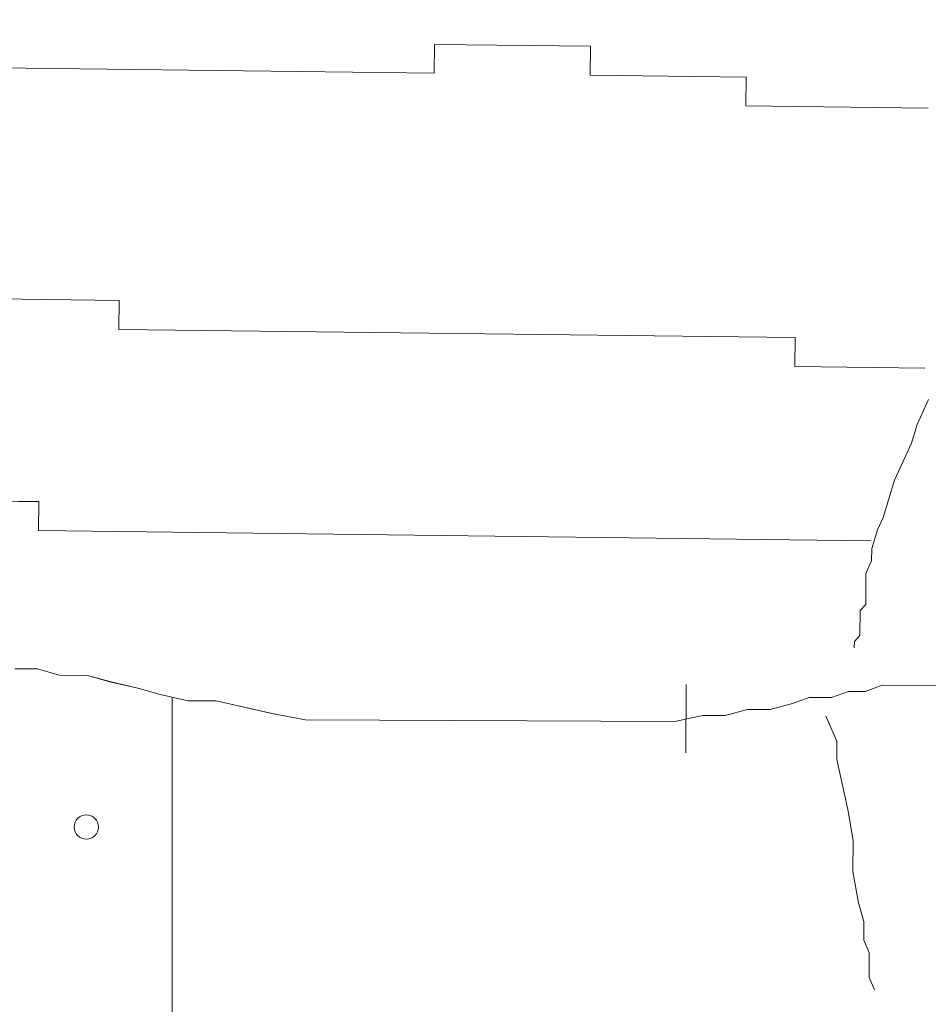
# Model space of a CAD drawing. Units: inches. Extents: x -466983 to 1020, y 324 to 318697.
# Tile 79 of 97: x 656.235 to 660.579, y 939.297 to 944.006. Entities that reach past the tile are written whole.
import ezdxf

# ---------------------------------------------------------------- set-up
doc = ezdxf.new("R2010")
doc.units = ezdxf.units.IN
doc.header["$MEASUREMENT"] = 0
doc.layers.add('A-FLOR-PATT', color=252, linetype='Continuous', lineweight=13)
doc.layers.add('A-FURN', color=8, linetype='Continuous', lineweight=18)

# ---------------------------------------------------------------- blocks, each defined once
blk = doc.blocks.new('L Shaped Sofa')
at = {"ltscale": 2}
for p, q in [((2394.7123, 747.2551), (2394.7123, 765.179)), ((2388.6357, 749.7), (2388.5876, 749.8086)), ((2388.6344, 749.4831), (2388.6357, 749.7)), ((2388.6826, 749.3745), (2388.6344, 749.4831)), ((2388.6816, 749.2118), (2388.6826, 749.3745)), ((2388.7294, 749.0489), (2388.6816, 749.2118)), ((2388.7765, 748.7776), (2388.7294, 749.0489)), ((2388.7748, 748.5065), (2388.7765, 748.7776)), ((2388.822, 748.2352), (2388.7748, 748.5065)), ((2388.9169, 747.801), (2388.822, 748.2352)), ((2388.9159, 747.6384), (2388.9169, 747.801)), ((2390.234, 747.7406), (2390.2304, 747.1443)), ((2389.0122, 747.4211), (2388.9159, 747.6384)), ((2390.0857, 747.416), (2390.33, 747.4691)), ((2390.33, 747.4691), (2393.5504, 747.454)), ((2393.5504, 747.454), (2393.8429, 747.3984)), ((2389.3043, 747.3113), (2389.4998, 747.3646)), ((2389.4998, 747.3646), (2389.695, 747.3637)), ((2389.695, 747.3637), (2389.8905, 747.417)), ((2389.8905, 747.417), (2390.0857, 747.416)), ((2393.8429, 747.3984), (2394.3302, 747.2877)), ((2389.1576, 747.2577), (2389.3043, 747.3113)), ((2394.3302, 747.2877), (2394.5741, 747.2865)), ((2394.5741, 747.2865), (2394.8178, 747.2312)), ((2388.5226, 747.1523), (2388.6693, 747.2058)), ((2388.6693, 747.2058), (2388.8157, 747.2051)), ((2388.8157, 747.2051), (2388.9624, 747.2587)), ((2388.9624, 747.2587), (2389.1576, 747.2577)), ((2394.8178, 747.2312), (2395.0126, 747.176)), ((2395.0126, 747.176), (2395.2563, 747.1207)), ((2387.3515, 747.1578), (2388.5226, 747.1523)), ((2395.2563, 747.1207), (2395.4511, 747.0656)), ((2395.4511, 747.0656), (2395.6951, 747.0644)), ((2395.6951, 747.0644), (2395.89, 747.0093)), ((2395.89, 747.0093), (2396.0851, 747.0084)), ((2388.7151, 746.7176), (2388.7642, 746.7716)), ((2388.7642, 746.7716), (2388.7645, 746.8258)), ((2388.7138, 746.5008), (2388.7151, 746.7176)), ((2388.6646, 746.4468), (2388.7138, 746.5008)), ((2388.663, 746.1757), (2388.6646, 746.4468)), ((2388.6135, 746.0675), (2388.663, 746.1757)), ((2388.6128, 745.9591), (2388.6135, 746.0675)), ((2388.5631, 745.7967), (2388.6128, 745.9591)), ((2388.6215, 745.891), (2395.8803, 745.8023)), ((2395.8803, 745.8023), (2395.8772, 745.5504)), ((2388.5136, 745.6885), (2388.5631, 745.7967)), ((2388.414, 745.3636), (2388.5136, 745.6885)), ((2395.8772, 745.5504), (2397.2382, 745.5337)), ((2388.2656, 745.039), (2388.414, 745.3636)), ((2388.2158, 744.8766), (2388.2656, 745.039)), ((2388.1169, 744.6602), (2388.2158, 744.8766)), ((2388.1494, 744.385), (2389.2836, 744.3712)), ((2389.2836, 744.3712), (2389.2805, 744.1193)), ((2389.2805, 744.1193), (2395.1782, 744.0472)), ((2395.1782, 744.0472), (2395.1752, 743.7953)), ((2395.1752, 743.7953), (2396.3094, 743.7814)), ((2388.1217, 742.1178), (2389.7096, 742.0984)), ((2389.7096, 742.0984), (2389.7065, 741.8465)), ((2389.7065, 741.8465), (2391.0675, 741.8299)), ((2391.0675, 741.8299), (2391.0644, 741.578)), ((2392.4254, 741.5613), (2392.4285, 741.8133)), ((2392.4285, 741.8133), (2397.6457, 741.7495)), ((2391.0644, 741.578), (2392.4254, 741.5613))]:
    blk.add_line(p, q, dxfattribs=at)
for start, end in [(90, 270), (270, 90)]:
    blk.add_arc((2395.4627, 748.3889), 0.1062, start, end, dxfattribs=at)

msp = doc.modelspace()

# ---------------------------------------------------------------- hatches: boundary and pattern name
at = {"layer": 'A-FLOR-PATT', "transparency": 33554572}
h = msp.add_hatch(dxfattribs=at)
h.set_pattern_fill('ANSI37', color=256, scale=30)
h.set_pattern_definition([(45, (-1212.4137, -290.035), (-2.6516504, 2.6516504), []), (135, (-1212.4137, -290.035), (-2.6516504, -2.6516504), [])])
h.paths.add_polyline_path([(901.8057, 1075.9377), (900.6144, 1075.9377), (900.6144, 1065.3856), (899.391, 1065.3856), (898.0911, 1065.3856), (892.8356, 1058.7098, -0.258377), (892.1875, 1058.3509), (879.9848, 1058.3509, -0.20177), (879.4382, 1058.5808), (874.0812, 1065.3856), (872.7813, 1065.3856), (871.5579, 1065.3856), (871.5579, 1075.9377), (813.8057, 1075.9377), (813.8057, 1044.7922), (832.3947, 1044.7922, -0.394795), (848.6602, 1028.5356), (848.6602, 1009.9377), (901.8057, 1009.9377), (901.8057, 1015.9377), (901.3057, 1015.9377), (871.3057, 1015.9377), (871.3057, 1017.2502), (871.3344, 1017.2502, -0.401453), (901.3057, 1045.9377), (901.8057, 1045.9377)])
edge = h.paths.add_edge_path(flags=16)
edge.add_line((847.7731, 1068.9486), (847.7731, 1073.7088))
edge.add_arc((849.2269, 1073.7088), 1.4538, 90, 180, ccw=False)
edge.add_line((849.2269, 1075.1627), (864.4921, 1075.1627))
edge.add_arc((864.4921, 1073.7088), 1.4538, 0, 90, ccw=False)
edge.add_line((865.9459, 1073.7088), (865.9459, 1069.0035))
edge.add_arc((832.6447, 1068.9761), 33.3012, -20.61234, 0.04725, ccw=False)
edge.add_ellipse((856.8595, 1058.48), major_axis=(0, 10.2131), ratio=0.6859192, start_angle=100.00884, end_angle=259.99116, ccw=False)
edge.add_arc((881.0742, 1068.9761), 33.3012, 180.04725, 200.61234, ccw=False)
h.paths.add_polyline_path([(853.1456, 1066.4815), (853.1456, 1066.4534), (853.1463, 1066.4534, 0.433107), (852.9166, 1066.6849), (852.9166, 1066.4534), (853.1456, 1066.4534), (853.1456, 1066.4815), (853.088, 1066.6122, 0.697939), (852.6995, 1066.4534), (852.7003, 1066.4534), (852.7003, 1066.4815), (852.9166, 1067.0012), (852.9166, 1066.6849, -0.396254)], flags=0)
h.paths.add_polyline_path([(861.0187, 1066.4815), (861.0187, 1066.4534), (861.0194, 1066.4534, 0.416404), (860.8024, 1066.6849), (860.8024, 1066.4534), (861.0187, 1066.4534), (861.0187, 1066.4815), (860.9672, 1066.6053, 0.713344), (860.5726, 1066.4534), (860.5734, 1066.4534), (860.5734, 1066.4815), (860.8024, 1067.0012), (860.8024, 1066.6849, -0.379973)], flags=0)
edge = h.paths.add_edge_path(flags=0)
edge.add_spline(control_points=[(861.1298, 1065.7855), (861.4661, 1065.2478), (861.6134, 1065.0161), (861.9833, 1064.3736), (862.1924, 1063.9443), (862.5614, 1063.0391), (862.7212, 1062.5633), (862.9865, 1061.5781), (863.092, 1061.0689), (863.2452, 1060.031), (863.293, 1059.5025), (863.3295, 1058.4409), (863.3181, 1057.9078), (863.2366, 1056.8518), (863.1664, 1056.3289), (862.9695, 1055.308), (862.8427, 1054.8099), (862.5365, 1053.8522), (862.3571, 1053.3927), (861.9514, 1052.5249), (861.7251, 1052.1166), (861.233, 1051.3622), (860.9672, 1051.0162), (860.4048, 1050.3949), (860.1082, 1050.1197), (859.4937, 1049.6461), (859.1758, 1049.4476), (858.5276, 1049.1299), (858.1973, 1049.0107), (857.5315, 1048.8518), (857.1959, 1048.8121), (856.5249, 1048.812), (856.1894, 1048.8515), (855.5236, 1049.0101), (855.1933, 1049.1291), (854.545, 1049.4465), (854.2271, 1049.6449), (853.6124, 1050.1183), (853.3158, 1050.3933), (852.7533, 1051.0143), (852.4874, 1051.3602), (851.9952, 1052.1144), (851.7688, 1052.5225), (851.3629, 1053.3902), (851.1834, 1053.8496), (850.877, 1054.8071), (850.7501, 1055.3051), (850.553, 1056.326), (850.4827, 1056.8488), (850.401, 1057.9048), (850.3895, 1058.4379), (850.4257, 1059.4995), (850.4734, 1060.0281), (850.6265, 1061.066), (850.7318, 1061.5753), (850.9969, 1062.5605), (851.1567, 1063.0365), (851.5254, 1063.9418), (851.7345, 1064.3712), (852.1056, 1065.0164), (852.2544, 1065.2503), (852.6082, 1065.7335)], knot_values=[3.915332, 3.915332, 3.915332, 3.915332, 4.013468, 4.013468, 4.175532, 4.175532, 4.337596, 4.337596, 4.49966, 4.49966, 4.661724, 4.661724, 4.823788, 4.823788, 4.985852, 4.985852, 5.147916, 5.147916, 5.30998, 5.30998, 5.472044, 5.472044, 5.634109, 5.634109, 5.796173, 5.796173, 5.958237, 5.958237, 6.120301, 6.120301, 6.282365, 6.282365, 6.444429, 6.444429, 6.606493, 6.606493, 6.768557, 6.768557, 6.930621, 6.930621, 7.092685, 7.092685, 7.254749, 7.254749, 7.416813, 7.416813, 7.578878, 7.578878, 7.740942, 7.740942, 7.903006, 7.903006, 8.06507, 8.06507, 8.227134, 8.227134, 8.389198, 8.389198, 8.551262, 8.551262, 8.65037, 8.65037, 8.65037, 8.65037], degree=3, periodic=0)
edge.add_line((852.6421, 1065.7855), (861.1298, 1065.7855))
edge = h.paths.add_edge_path(flags=0)
edge.add_ellipse((856.8496, 1057.7432), major_axis=(0, 7.7921), ratio=0.687861, start_angle=0, end_angle=360)
h.paths.add_polyline_path([(848.8634, 1069.3891), (848.8634, 1073.9605, -0.414214), (849.9538, 1075.0508), (863.7652, 1075.0508, -0.414214), (864.8555, 1073.9605), (864.8555, 1069.3891, -0.388936), (864.5237, 1069.027, -0.043561), (849.1953, 1069.027, -0.388936)], flags=0)
h.paths.add_polyline_path([(853.1006, 1068.1122, -1), (852.6775, 1068.1122, -1)], flags=0)
edge = h.paths.add_edge_path(flags=0)
edge.add_ellipse((856.8595, 1057.3378), major_axis=(0, 2.207), ratio=0.657164, start_angle=0, end_angle=360)
h.paths.add_polyline_path([(861.0415, 1068.1122, -1), (860.6184, 1068.1122, -1)], flags=0)
edge = h.paths.add_edge_path()
edge.add_line((573.9537, 1057.3412), (573.9537, 1075.9377))
edge.add_line((573.9537, 1075.9377), (558.7308, 1075.9377))
edge.add_line((558.7308, 1075.9377), (558.7308, 1065.3856))
edge.add_line((558.7308, 1065.3856), (557.5074, 1065.3856))
edge.add_line((557.5074, 1065.3856), (556.2075, 1065.3856))
edge.add_line((556.2075, 1065.3856), (550.952, 1058.7098))
edge.add_arc((550.3039, 1059.1155), 0.7646, 270, 327.9483, ccw=False)
edge.add_line((550.3039, 1058.3509), (538.1012, 1058.3509))
edge.add_arc((538.1012, 1059.1155), 0.7646, 224.3704, 270, ccw=False)
edge.add_line((537.5546, 1058.5808), (532.1976, 1065.3856))
edge.add_line((532.1976, 1065.3856), (530.8977, 1065.3856))
edge.add_line((530.8977, 1065.3856), (529.6743, 1065.3856))
edge.add_line((529.6743, 1065.3856), (529.6743, 1075.9377))
edge.add_line((529.6743, 1075.9377), (520.8057, 1075.9377))
edge.add_line((520.8057, 1075.9377), (520.8057, 1045.9377))
edge.add_line((520.8057, 1045.9377), (521.3057, 1045.9377))
edge.add_arc((521.3057, 1015.9377), 30, 2.50749, 90, ccw=False)
edge.add_line((551.277, 1017.2502), (551.3057, 1017.2502))
edge.add_line((551.3057, 1017.2502), (551.3057, 1015.9377))
edge.add_line((551.3057, 1015.9377), (520.8057, 1015.9377))
edge.add_line((520.8057, 1015.9377), (520.8057, 1009.9377))
edge.add_line((520.8057, 1009.9377), (559.1913, 1010.4022))
edge.add_arc((559.1913, 1011.856), 1.4538, 180, 270, ccw=False)
edge.add_line((557.7375, 1011.856), (557.7375, 1016.5613))
edge.add_arc((591.0386, 1016.5888), 33.3012, 159.38766, 180.04725, ccw=False)
edge.add_ellipse((566.8239, 1027.0848), major_axis=(0, 10.2131), ratio=0.6859192, start_angle=280.00884, end_angle=439.99116, ccw=False)
edge.add_arc((542.6091, 1016.5888), 33.3012, 0.04725, 20.61234, ccw=False)
edge.add_line((575.9103, 1016.6162), (575.9103, 1011.856))
edge.add_arc((574.4565, 1011.856), 1.4538, -90, 0, ccw=False)
edge.add_line((574.4565, 1010.4022), (608.8057, 1009.9377))
edge.add_line((608.8057, 1009.9377), (608.8057, 1041.0857))
edge.add_line((608.8057, 1041.0857), (590.2179, 1041.0857))
edge.add_arc((590.775, 1057.9074), 16.8309, 181.92775, 268.10321, ccw=False)
edge = h.paths.add_edge_path()
edge.add_ellipse((494.2443, 583.6204), major_axis=(0, 10.2131), ratio=0.6859192, start_angle=280.00884, end_angle=439.99116, ccw=False)
edge.add_arc((470.0296, 573.1243), 33.3012, 0.04725, 20.61234, ccw=False)
edge.add_line((503.3307, 573.1518), (503.3307, 568.3916))
edge.add_arc((501.8769, 568.3916), 1.4538, -90, 0, ccw=False)
edge.add_line((501.8769, 566.9377), (539.8057, 566.9377))
edge.add_line((539.8057, 566.9377), (539.8057, 572.9377))
edge.add_line((539.8057, 572.9377), (539.3057, 572.9377))
edge.add_line((539.3057, 572.9377), (509.3057, 572.9377))
edge.add_line((509.3057, 572.9377), (509.3057, 574.2502))
edge.add_line((509.3057, 574.2502), (509.3344, 574.2502))
edge.add_arc((539.3057, 572.9377), 30, 90, 177.49251, ccw=False)
edge.add_line((539.3057, 602.9377), (539.8057, 602.9377))
edge.add_line((539.8057, 602.9377), (539.8057, 626.9377))
edge.add_line((539.8057, 626.9377), (531.7718, 626.9377))
edge.add_line((531.7718, 626.9377), (531.7718, 616.3856))
edge.add_line((531.7718, 616.3856), (530.5484, 616.3856))
edge.add_line((530.5484, 616.3856), (529.2485, 616.3856))
edge.add_line((529.2485, 616.3856), (523.7105, 609.3509))
edge.add_line((523.7105, 609.3509), (510.7766, 609.3509))
edge.add_line((510.7766, 609.3509), (505.2386, 616.3856))
edge.add_line((505.2386, 616.3856), (503.9387, 616.3856))
edge.add_line((503.9387, 616.3856), (502.7153, 616.3856))
edge.add_line((502.7153, 616.3856), (502.7153, 626.9377))
edge.add_line((502.7153, 626.9377), (481.6983, 626.9377))
edge.add_line((481.6983, 626.9377), (481.6983, 610.995))
edge.add_arc((467.2703, 611.4728), 14.4359, 271.92775, 358.10321, ccw=False)
edge.add_line((467.7559, 597.0451), (451.8057, 597.0451))
edge.add_line((451.8057, 597.0451), (451.8057, 584.4035))
edge.add_line((451.8057, 584.4035), (451.8057, 566.9377))
edge.add_line((451.8057, 566.9377), (486.6117, 566.9377))
edge.add_arc((486.6117, 568.3916), 1.4538, 180, 270, ccw=False)
edge.add_line((485.1579, 568.3916), (485.1579, 573.0969))
edge.add_arc((518.4591, 573.1243), 33.3012, 159.38766, 180.04725, ccw=False)
h.paths.add_polyline_path([(836.2609, 1020.7328), (879.8898, 1020.7328), (879.8898, 1039.3902), (836.2609, 1039.3902)], flags=25)
h.paths.add_polyline_path([(549.9851, 1036.7492), (593.614, 1036.7492), (593.614, 1055.4065), (549.9851, 1055.4065)], flags=24)
h.paths.add_polyline_path([(475.123, 595.5959), (518.752, 595.5959), (518.752, 614.2532), (475.123, 614.2532)], flags=24)
h = msp.add_hatch(dxfattribs=at)
h.set_pattern_fill('ANSI37', color=256, scale=20)
h.set_pattern_definition([(45, (-1212.4137, -290.035), (-1.767767, 1.767767), []), (135, (-1212.4137, -290.035), (-1.767767, -1.767767), [])])
h.paths.add_polyline_path([(809.8057, 870.9377), (809.8057, 888.1519), (806.9985, 888.1519), (802.6624, 888.1519), (789.3832, 888.1519), (786.2846, 888.1519, -0.414214), (785.4991, 888.9374), (785.4991, 900.1959), (785.4991, 908.4696, -0.414214), (786.8082, 909.7787, -0.414214), (785.4991, 911.0878), (785.4991, 929.1015, -0.414214), (786.8082, 930.4106, -0.414214), (785.4991, 931.7197), (785.4991, 931.9039, -0.414214), (784.19, 930.5948), (766.7223, 930.5948, -0.412359), (765.4132, 931.8956, -0.413741), (764.1145, 930.5782), (744.5781, 930.422, -0.416556), (743.7864, 931.2075), (743.7864, 933.5153), (742.2154, 933.5153), (742.2154, 952.024, -0.001344), (743.7864, 952.1998), (743.7864, 953.9377), (678.5915, 953.9377), (678.5915, 951.1305), (678.5915, 946.7945), (678.5915, 933.5153), (678.5915, 930.4166, -0.414214), (677.806, 929.6312), (666.5475, 929.6312), (658.2738, 929.6312, -0.414214), (656.9647, 930.9403, -0.414214), (655.6556, 929.6312), (637.6419, 929.6312, -0.414214), (636.3328, 930.9403, -0.414214), (635.0237, 929.6312), (634.8395, 929.6312, -0.414214), (636.1486, 928.322), (636.1486, 910.8544, -0.412359), (634.8478, 909.5452, -0.413741), (636.1653, 908.2466), (636.3214, 888.7102, -0.416556), (635.5359, 887.9184), (633.2281, 887.9184), (633.2281, 886.3475), (614.7194, 886.3475, -0.001344), (614.5436, 887.9184), (612.8057, 887.9184), (612.8057, 834.9377), (612.8057, 752.9377), (612.8057, 748.9377), (612.8057, 697.9377), (654.8057, 697.9377), (654.8057, 701.9377), (715.8057, 701.9377), (715.8057, 737.4353), (774.2918, 737.4353), (774.2918, 795.9377), (809.8057, 795.9377)])
h.paths.add_polyline_path([(679.2761, 849.5757, 0.102523), (682.1475, 849.2608, -0.080461), (694.5428, 849.7725, -0.283899), (694.4822, 849.0082, 0.136605), (694.4068, 848.8103, -0.030441), (694.5428, 846.8929), (694.5428, 842.6198), (694.5428, 838.3466, -0.028219), (694.4246, 836.5684), (694.425, 836.5684, 0.196187), (694.4456, 836.2708, -0.302897), (694.5428, 835.467, -0.080461), (682.1475, 835.9787, 0.102523), (679.2761, 835.6638, -0.58611), (678.6457, 836.0169), (678.6457, 849.2227, -0.58611)], flags=16)
h.paths.add_polyline_path([(679.5173, 848.6515, 0.699597), (679.476, 848.6342, 1.20716), (679.1935, 848.7422, 0.010621)], flags=0)
h.paths.add_polyline_path([(679.4923, 836.5608, -0.013798), (679.9178, 836.6594, -0.071703), (682.8533, 837.1434, -0.165743), (682.1665, 839.1006), (682.1665, 842.6094), (682.1665, 846.0603, -0.240616), (683.4733, 848.6767, -0.068263), (693.9295, 849.0082), (693.7875, 848.7083), (693.7875, 849.0228, 0.067332), (683.4733, 848.6767, 0.240616), (682.1665, 846.0603), (682.1665, 842.6094), (682.1665, 839.1006, 0.23459), (683.461, 836.5513, 0.068093), (693.7875, 836.1955), (693.7875, 836.5104), (693.9296, 836.2102, -0.077215), (682.2421, 836.7815, 0.086627), (679.5283, 836.5701, -0.628402), (679.5029, 836.5735), (679.5029, 836.6071, 0.910458)], flags=0)
h.paths.add_polyline_path([(679.476, 848.6364), (679.2069, 848.647), (679.2069, 836.5718, 0.913566), (679.3645, 836.5861), (679.476, 836.5824)], flags=0)
h.paths.add_polyline_path([(679.2761, 829.8604, 0.102523), (682.1475, 829.5455, -0.080461), (694.5428, 830.0572, -0.283899), (694.4822, 829.2929, 0.136605), (694.4068, 829.095, -0.030441), (694.5428, 827.1776), (694.5428, 822.9045), (694.5428, 818.6314, -0.028219), (694.4246, 816.8531), (694.425, 816.8532, 0.196187), (694.4456, 816.5555, -0.302897), (694.5428, 815.7517, -0.080461), (682.1475, 816.2635, 0.102523), (679.2761, 815.9485, -0.58611), (678.6457, 816.3016), (678.6457, 829.5074, -0.58611)], flags=16)
h.paths.add_polyline_path([(679.5173, 828.9362, 0.699597), (679.476, 828.9189, 1.20716), (679.1935, 829.0269, 0.010621)], flags=0)
h.paths.add_polyline_path([(679.4923, 816.8456, -0.013798), (679.9178, 816.9441, -0.071703), (682.8533, 817.4281, -0.165743), (682.1665, 819.3853), (682.1665, 822.8941), (682.1665, 826.345, -0.240616), (683.4733, 828.9614, -0.068263), (693.9295, 829.2929), (693.7875, 828.9931), (693.7875, 829.3076, 0.067332), (683.4733, 828.9614, 0.240616), (682.1665, 826.345), (682.1665, 822.8941), (682.1665, 819.3853, 0.23459), (683.461, 816.836, 0.068093), (693.7875, 816.4802), (693.7875, 816.7952), (693.9296, 816.4949, -0.077215), (682.2421, 817.0662, 0.086627), (679.5283, 816.8549, -0.628402), (679.5029, 816.8582), (679.5029, 816.8918, 0.910458)], flags=0)
h.paths.add_polyline_path([(679.476, 828.9211), (679.2069, 828.9317), (679.2069, 816.8565, 0.913566), (679.3645, 816.8708), (679.476, 816.8671)], flags=0)
h.paths.add_polyline_path([(679.2761, 810.1451, 0.102523), (682.1475, 809.8302, -0.080461), (694.5428, 810.342, -0.3023), (694.4466, 809.5394, 0.10023), (694.4058, 809.3878, -0.03057), (694.5428, 807.4623), (694.5428, 803.1892), (694.5428, 798.9161, -0.03057), (694.4058, 796.9906, 0.10023), (694.4466, 796.839, -0.3023), (694.5428, 796.0365, -0.080461), (682.1475, 796.5482, 0.102523), (679.2761, 796.2333, -0.58611), (678.6457, 796.5863), (678.6457, 809.7921, -0.58611)], flags=16)
h.paths.add_polyline_path([(679.5173, 809.2417, 0.699597), (679.476, 809.2244, 1.20716), (679.1935, 809.3324, 0.010621)], flags=0)
h.paths.add_polyline_path([(679.4923, 797.151, -0.013798), (679.9178, 797.2496, -0.071703), (682.8533, 797.7336, -0.165743), (682.1665, 799.6908), (682.1665, 803.1996), (682.1665, 806.6505, -0.239349), (683.461, 809.2577, -0.072465), (694.4468, 809.5405, 0.197932), (694.425, 809.2405), (693.7875, 809.2985), (693.7875, 809.6135, 0.068093), (683.461, 809.2577, 0.239349), (682.1665, 806.6505), (682.1665, 803.1996), (682.1665, 799.6908, 0.235854), (683.4733, 797.1323, 0.067332), (693.7875, 796.7861), (693.7875, 797.1006), (694.425, 797.1586, 0.197932), (694.4468, 796.8586, -0.080419), (682.1557, 797.3795, 0.083867), (679.5283, 797.1603, -0.628402), (679.5029, 797.1637), (679.5029, 797.1973, 0.910458)], flags=0)
h.paths.add_polyline_path([(679.2069, 809.2372), (679.2069, 797.162, 0.913566), (679.3645, 797.1763), (679.476, 797.1726), (679.476, 809.2266)], flags=0)
h.paths.add_polyline_path([(695.3643, 853.2989), (728.2231, 853.2989), (728.2231, 771.1519), (695.3643, 771.1519)], flags=16)
h.paths.add_polyline_path([(696.0215, 852.6417), (727.5659, 852.6417), (727.5659, 771.809), (696.0215, 771.809)], flags=0)
h.paths.add_polyline_path([(679.2761, 788.7869, 0.102523), (682.1475, 788.472, -0.080461), (694.5428, 788.9837, -0.3023), (694.4466, 788.1812, 0.10023), (694.4058, 788.0296, -0.03057), (694.5428, 786.1041), (694.5428, 781.831), (694.5428, 777.5578, -0.03057), (694.4058, 775.6323, 0.10023), (694.4466, 775.4808, -0.3023), (694.5428, 774.6782, -0.080461), (682.1475, 775.19, 0.102523), (679.2761, 774.875, -0.58611), (678.6457, 775.2281), (678.6457, 788.4339, -0.58611)], flags=16)
h.paths.add_polyline_path([(679.5173, 787.8834, 0.699597), (679.476, 787.8662, 1.20716), (679.1935, 787.9742, 0.010621)], flags=0)
h.paths.add_polyline_path([(679.4923, 775.7928, -0.013798), (679.9178, 775.8914, -0.071703), (682.8533, 776.3753, -0.165743), (682.1665, 778.3325), (682.1665, 781.8414), (682.1665, 785.2922, -0.239349), (683.461, 787.8995, -0.072465), (694.4468, 788.1823, 0.197932), (694.425, 787.8823), (693.7875, 787.9403), (693.7875, 788.2553, 0.068093), (683.461, 787.8995, 0.239349), (682.1665, 785.2922), (682.1665, 781.8414), (682.1665, 778.3325, 0.235854), (683.4733, 775.7741, 0.067332), (693.7875, 775.4279), (693.7875, 775.7424), (694.425, 775.8004, 0.197932), (694.4468, 775.5004, -0.080419), (682.1557, 776.0212, 0.083867), (679.5283, 775.8021, -0.628402), (679.5029, 775.8054), (679.5029, 775.8391, 0.910458)], flags=0)
h.paths.add_polyline_path([(679.2069, 787.8789), (679.2069, 775.8038, 0.913566), (679.3645, 775.818), (679.476, 775.8144), (679.476, 787.8684)], flags=0)
h.paths.add_polyline_path([(704.641, 854.1204, -0.080461), (705.1527, 866.5157, 0.102523), (704.8378, 869.3871, -0.58611), (705.1908, 870.0174), (718.3966, 870.0174, -0.58611), (718.7496, 869.3871, 0.102523), (718.4347, 866.5157, -0.080461), (718.9465, 854.1204, -0.3023), (718.1439, 854.2166, 0.10023), (717.9924, 854.2574, -0.03057), (716.0668, 854.1204), (711.7937, 854.1204), (707.5206, 854.1204, -0.03057), (705.5951, 854.2574, 0.10023), (705.4435, 854.2166, -0.3023)], flags=16)
h.paths.add_polyline_path([(717.8462, 869.1459, 0.699597), (717.8289, 869.1872, 1.20716), (717.9369, 869.4697, 0.010621)], flags=0)
h.paths.add_polyline_path([(705.4631, 854.2164, -0.080419), (705.984, 866.5074, 0.083867), (705.7648, 869.1349, -0.628402), (705.7682, 869.1603), (705.8018, 869.1603, 0.910458), (705.7555, 869.1709, -0.013798), (705.8541, 868.7454, -0.071703), (706.3381, 865.8099, -0.165743), (708.2953, 866.4967), (711.8041, 866.4967), (715.255, 866.4967, -0.239349), (717.8622, 865.2022, -0.072465), (718.145, 854.2164, 0.197932), (717.845, 854.2382), (717.903, 854.8757), (718.218, 854.8757, 0.068093), (717.8622, 865.2022, 0.239349), (715.255, 866.4967), (711.8041, 866.4967), (708.2953, 866.4967, 0.235854), (705.7368, 865.1898, 0.067332), (705.3906, 854.8757), (705.7051, 854.8757), (705.7631, 854.2382, 0.197932)], flags=16)
h.paths.add_polyline_path([(705.7665, 869.4563, 0.913566), (705.7808, 869.2987), (705.7771, 869.1872), (717.8311, 869.1872), (717.8417, 869.4563)], flags=0)
h.paths.add_polyline_path([(729.0446, 842.6198), (729.0446, 846.8929, -0.03057), (729.1817, 848.8184, 0.10023), (729.1408, 848.9699, -0.3023), (729.0446, 849.7725, -0.080461), (741.4399, 849.2608, 0.102523), (744.3113, 849.5757, -0.58611), (744.9417, 849.2227), (744.9417, 836.0169, -0.58611), (744.3113, 835.6638, 0.102523), (741.4399, 835.9787, -0.080461), (729.0446, 835.467, -0.3023), (729.1408, 836.2696, 0.10023), (729.1817, 836.4211, -0.03057), (729.0446, 838.3466)], flags=16)
h.paths.add_polyline_path([(744.1115, 836.5846, 1.20716), (744.3939, 836.4766, 0.010621), (744.0701, 836.5673, 0.699597)], flags=0)
h.paths.add_polyline_path([(729.1407, 836.2684, 0.197932), (729.1624, 836.5684), (729.7999, 836.5104), (729.7999, 836.1955, 0.068093), (740.1264, 836.5513, 0.239349), (741.4209, 839.1585), (741.4209, 842.6094), (741.4209, 846.1182, 0.235854), (740.1141, 848.6767, 0.067332), (729.7999, 849.0228), (729.7999, 848.7083), (729.1624, 848.6503, 0.197932), (729.1407, 848.9504, -0.080419), (741.4317, 848.4295, 0.083867), (744.0591, 848.6486, -0.628402), (744.0845, 848.6453), (744.0845, 848.6117, 0.910458), (744.0951, 848.6579, -0.013798), (743.6696, 848.5594, -0.071703), (740.7341, 848.0754, -0.165743), (741.4209, 846.1182), (741.4209, 842.6094), (741.4209, 839.1585, -0.239349), (740.1264, 836.5513, -0.072465)], flags=0)
h.paths.add_polyline_path([(729.0446, 830.0572, -0.080461), (741.4399, 829.5455, 0.102523), (744.3113, 829.8604, -0.58611), (744.9417, 829.5074), (744.9417, 816.3016, -0.58611), (744.3113, 815.9485, 0.102523), (741.4399, 816.2635, -0.080461), (729.0446, 815.7517, -0.3023), (729.1408, 816.5543, 0.10023), (729.1817, 816.7058, -0.03057), (729.0446, 818.6314), (729.0446, 822.9045), (729.0446, 827.1776, -0.03057), (729.1817, 829.1031, 0.10023), (729.1408, 829.2547, -0.3023)], flags=16)
h.paths.add_polyline_path([(744.1115, 816.8693, 1.20716), (744.3939, 816.7613, 0.010621), (744.0701, 816.852, 0.699597)], flags=0)
h.paths.add_polyline_path([(729.1407, 829.2351, -0.080419), (741.4317, 828.7142, 0.083867), (744.0591, 828.9334, -0.628402), (744.0845, 828.93), (744.0845, 828.8964, 0.910458), (744.0951, 828.9427, -0.013798), (743.6696, 828.8441, -0.071703), (740.7341, 828.3601, -0.165743), (741.4209, 826.4029), (741.4209, 822.8941), (741.4209, 819.4432, -0.239349), (740.1264, 816.836, -0.072465), (729.1407, 816.5531, 0.197932), (729.1624, 816.8532), (729.7999, 816.7952), (729.7999, 816.4802, 0.068093), (740.1264, 816.836, 0.239349), (741.4209, 819.4432), (741.4209, 822.8941), (741.4209, 826.4029, 0.235854), (740.1141, 828.9614, 0.067332), (729.7999, 829.3076), (729.7999, 828.9931), (729.1624, 828.9351, 0.197932)], flags=16)
h.paths.add_polyline_path([(729.0446, 810.342, -0.080461), (741.4399, 809.8302, 0.102523), (744.3113, 810.1451, -0.58611), (744.9417, 809.7921), (744.9417, 796.5863, -0.58611), (744.3113, 796.2333, 0.102523), (741.4399, 796.5482, -0.080461), (729.0446, 796.0365, -0.283899), (729.1052, 796.8007, 0.136605), (729.1806, 796.9987, -0.030441), (729.0446, 798.9161), (729.0446, 803.1892), (729.0446, 807.4623, -0.028219), (729.1628, 809.2406), (729.1624, 809.2405, 0.196187), (729.1418, 809.5382, -0.302897)], flags=16)
h.paths.add_polyline_path([(744.1115, 797.1748, 1.20716), (744.3939, 797.0668, 0.010621), (744.0701, 797.1575, 0.699597)], flags=0)
h.paths.add_polyline_path([(741.3453, 809.0275, 0.086627), (744.0591, 809.2388, -0.628402), (744.0845, 809.2355), (744.0845, 809.2019, 0.910458), (744.0951, 809.2481, -0.013798), (743.6696, 809.1496, -0.071703), (740.7341, 808.6656, -0.165743), (741.4209, 806.7084), (741.4209, 803.1996), (741.4209, 799.7487, -0.240616), (740.1141, 797.1323, -0.068263), (729.658, 796.8008), (729.7999, 797.1006), (729.7999, 796.7861, 0.067332), (740.1141, 797.1323, 0.240616), (741.4209, 799.7487), (741.4209, 803.1996), (741.4209, 806.7084, 0.23459), (740.1264, 809.2577, 0.068093), (729.7999, 809.6135), (729.7999, 809.2985), (729.6578, 809.5988, -0.077215)], flags=0)
h.paths.add_polyline_path([(704.641, 770.3304, -0.283899), (705.4053, 770.2697, 0.136605), (705.6032, 770.1944, -0.030441), (707.5206, 770.3304), (711.7937, 770.3304), (716.0668, 770.3304, -0.028219), (717.8451, 770.2122), (717.845, 770.2126, 0.196187), (718.1427, 770.2331, -0.302897), (718.9465, 770.3304, -0.080461), (718.4347, 757.9351, 0.102523), (718.7496, 755.0637, -0.58611), (718.3966, 754.4333), (705.1908, 754.4333, -0.58611), (704.8378, 755.0637, 0.102523), (705.1527, 757.9351, -0.080461)], flags=16)
h.paths.add_polyline_path([(705.762, 755.3048, 0.699597), (705.7793, 755.2635, 1.20716), (705.6713, 754.9811, 0.010621)], flags=0)
h.paths.add_polyline_path([(705.4053, 769.717), (705.7051, 769.5751), (705.3906, 769.5751, 0.067332), (705.7368, 759.2609, 0.240616), (708.3532, 757.954), (711.8041, 757.954), (715.3129, 757.954, 0.23459), (717.8622, 759.2485, 0.068093), (718.218, 769.5751), (717.903, 769.5751), (718.2033, 769.7172, -0.077215), (717.632, 758.0297, 0.086627), (717.8433, 755.3159, -0.628402), (717.84, 755.2904), (717.8064, 755.2904, 0.910458), (717.8526, 755.2799, -0.013798), (717.7541, 755.7053, -0.071703), (717.2701, 758.6409, -0.165743), (715.3129, 757.954), (711.8041, 757.954), (708.3532, 757.954, -0.240616), (705.7368, 759.2609, -0.068263)], flags=0)
h.paths.add_polyline_path([(729.0446, 788.9837, -0.080461), (741.4399, 788.472, 0.102523), (744.3113, 788.7869, -0.58611), (744.9417, 788.4339), (744.9417, 775.2281, -0.58611), (744.3113, 774.875, 0.102523), (741.4399, 775.19, -0.080461), (729.0446, 774.6782, -0.283899), (729.1052, 775.4425, 0.136605), (729.1806, 775.6405, -0.030441), (729.0446, 777.5578), (729.0446, 781.831), (729.0446, 786.1041, -0.028219), (729.1628, 787.8823), (729.1624, 787.8823, 0.196187), (729.1418, 788.1799, -0.302897)], flags=16)
h.paths.add_polyline_path([(744.1115, 775.8165, 1.20716), (744.3939, 775.7086, 0.010621), (744.0701, 775.7993, 0.699597)], flags=0)
h.paths.add_polyline_path([(741.3453, 787.6692, 0.086627), (744.0591, 787.8806, -0.628402), (744.0845, 787.8773), (744.0845, 787.8437, 0.910458), (744.0951, 787.8899, -0.013798), (743.6696, 787.7913, -0.071703), (740.7341, 787.3074, -0.165743), (741.4209, 785.3502), (741.4209, 781.8414), (741.4209, 778.3905, -0.240616), (740.1141, 775.7741, -0.068263), (729.658, 775.4425), (729.7999, 775.7424), (729.7999, 775.4279, 0.067332), (740.1141, 775.7741, 0.240616), (741.4209, 778.3905), (741.4209, 781.8414), (741.4209, 785.3502, 0.23459), (740.1264, 787.8995, 0.068093), (729.7999, 788.2553), (729.7999, 787.9403), (729.6578, 788.2405, -0.077215)], flags=0)
h.paths.add_polyline_path([(744.1115, 848.6364), (744.1115, 836.5824), (744.3805, 836.5718), (744.3805, 848.647, 0.913566), (744.2229, 848.6327)], flags=0)
h.paths.add_polyline_path([(744.2229, 828.9174), (744.1115, 828.9211), (744.1115, 816.8671), (744.3805, 816.8565), (744.3805, 828.9317, 0.913566)], flags=0)
h.paths.add_polyline_path([(717.8311, 755.2635), (705.7771, 755.2635), (705.7665, 754.9945), (717.8417, 754.9945, 0.913566), (717.8274, 755.1521)], flags=0)
h.paths.add_polyline_path([(744.2229, 809.2229), (744.1115, 809.2266), (744.1115, 797.1726), (744.3805, 797.162), (744.3805, 809.2372, 0.913566)], flags=0)
h.paths.add_polyline_path([(744.1115, 787.8684), (744.1115, 775.8144), (744.3805, 775.8038), (744.3805, 787.8789, 0.913566), (744.2229, 787.8647)], flags=0)
h.paths.add_polyline_path([(678.8774, 877.1228), (737.6127, 877.1228), (737.6127, 899.5116), (678.8774, 899.5116)], flags=24)

# ---------------------------------------------------------------- linework, layer by layer
at = {"layer": 'A-FURN', "ltscale": 2}
for p, q in [((658.2184, 943.8879), (658.2167, 943.7498)), ((658.2184, 943.8879), (658.2167, 943.7498)), ((658.2184, 943.8879), (658.2167, 943.7498)), ((658.2184, 943.8879), (658.2167, 943.7498)), ((658.2184, 943.8879), (658.2167, 943.7498)), ((658.2184, 943.8879), (658.2167, 943.7498)), ((658.9645, 943.8788), (658.2184, 943.8879)), ((658.9645, 943.8788), (658.2184, 943.8879)), ((658.9645, 943.8788), (658.2184, 943.8879)), ((658.9645, 943.8788), (658.2184, 943.8879)), ((658.9645, 943.8788), (658.2184, 943.8879)), ((658.9645, 943.8788), (658.2184, 943.8879)), ((658.9628, 943.7407), (658.9645, 943.8788)), ((658.9628, 943.7407), (658.9645, 943.8788)), ((658.9628, 943.7407), (658.9645, 943.8788)), ((658.9628, 943.7407), (658.9645, 943.8788)), ((658.9628, 943.7407), (658.9645, 943.8788)), ((658.9628, 943.7407), (658.9645, 943.8788)), ((658.2167, 943.7498), (655.3565, 943.7847)), ((658.2167, 943.7498), (655.3565, 943.7847)), ((658.2167, 943.7498), (655.3565, 943.7847)), ((658.2167, 943.7498), (655.3565, 943.7847)), ((658.2167, 943.7498), (655.3565, 943.7847)), ((658.2167, 943.7498), (655.3565, 943.7847)), ((659.709, 943.7315), (658.9628, 943.7407)), ((659.709, 943.7315), (658.9628, 943.7407)), ((659.709, 943.7315), (658.9628, 943.7407)), ((659.709, 943.7315), (658.9628, 943.7407)), ((659.709, 943.7315), (658.9628, 943.7407)), ((659.709, 943.7315), (658.9628, 943.7407)), ((659.7073, 943.5934), (659.709, 943.7315)), ((659.7073, 943.5934), (659.709, 943.7315)), ((659.7073, 943.5934), (659.709, 943.7315)), ((659.7073, 943.5934), (659.709, 943.7315)), ((659.7073, 943.5934), (659.709, 943.7315)), ((659.7073, 943.5934), (659.709, 943.7315)), ((660.5778, 943.5828), (659.7073, 943.5934)), ((660.5778, 943.5828), (659.7073, 943.5934)), ((660.5778, 943.5828), (659.7073, 943.5934)), ((660.5778, 943.5828), (659.7073, 943.5934)), ((660.5778, 943.5828), (659.7073, 943.5934)), ((660.5778, 943.5828), (659.7073, 943.5934)), ((656.711, 942.6632), (656.0892, 942.6708)), ((656.711, 942.6632), (656.0892, 942.6708)), ((656.711, 942.6632), (656.0892, 942.6708)), ((656.711, 942.6632), (656.0892, 942.6708)), ((656.711, 942.6632), (656.0892, 942.6708)), ((656.711, 942.6632), (656.0892, 942.6708)), ((656.7093, 942.5251), (656.711, 942.6632)), ((656.7093, 942.5251), (656.711, 942.6632)), ((656.7093, 942.5251), (656.711, 942.6632)), ((656.7093, 942.5251), (656.711, 942.6632)), ((656.7093, 942.5251), (656.711, 942.6632)), ((656.7093, 942.5251), (656.711, 942.6632)), ((659.9425, 942.4856), (656.7093, 942.5251)), ((659.9425, 942.4856), (656.7093, 942.5251)), ((659.9425, 942.4856), (656.7093, 942.5251)), ((659.9425, 942.4856), (656.7093, 942.5251)), ((659.9425, 942.4856), (656.7093, 942.5251)), ((659.9425, 942.4856), (656.7093, 942.5251)), ((659.9408, 942.3475), (659.9425, 942.4856)), ((659.9408, 942.3475), (659.9425, 942.4856)), ((659.9408, 942.3475), (659.9425, 942.4856)), ((659.9408, 942.3475), (659.9425, 942.4856)), ((659.9408, 942.3475), (659.9425, 942.4856)), ((659.9408, 942.3475), (659.9425, 942.4856)), ((660.5626, 942.3399), (659.9408, 942.3475)), ((660.5626, 942.3399), (659.9408, 942.3475)), ((660.5626, 942.3399), (659.9408, 942.3475)), ((660.5626, 942.3399), (659.9408, 942.3475)), ((660.5626, 942.3399), (659.9408, 942.3475)), ((660.5626, 942.3399), (659.9408, 942.3475)), ((660.5804, 942.189), (660.5262, 942.0704)), ((660.5804, 942.189), (660.5262, 942.0704)), ((660.5804, 942.189), (660.5262, 942.0704)), ((660.5804, 942.189), (660.5262, 942.0704)), ((660.5804, 942.189), (660.5262, 942.0704)), ((660.5804, 942.189), (660.5262, 942.0704)), ((660.5262, 942.0704), (660.4989, 941.9814)), ((660.5262, 942.0704), (660.4989, 941.9814)), ((660.5262, 942.0704), (660.4989, 941.9814)), ((660.5262, 942.0704), (660.4989, 941.9814)), ((660.5262, 942.0704), (660.4989, 941.9814)), ((660.5262, 942.0704), (660.4989, 941.9814)), ((660.4989, 941.9814), (660.4175, 941.8034)), ((660.4989, 941.9814), (660.4175, 941.8034)), ((660.4989, 941.9814), (660.4175, 941.8034)), ((660.4989, 941.9814), (660.4175, 941.8034)), ((660.4989, 941.9814), (660.4175, 941.8034)), ((660.4989, 941.9814), (660.4175, 941.8034)), ((660.4175, 941.8034), (660.3629, 941.6253)), ((660.4175, 941.8034), (660.3629, 941.6253)), ((660.4175, 941.8034), (660.3629, 941.6253)), ((660.4175, 941.8034), (660.3629, 941.6253)), ((660.4175, 941.8034), (660.3629, 941.6253)), ((660.4175, 941.8034), (660.3629, 941.6253)), ((656.3261, 941.701), (655.5799, 941.7102)), ((656.3261, 941.701), (655.5799, 941.7102)), ((656.3261, 941.701), (655.5799, 941.7102)), ((656.3261, 941.701), (655.5799, 941.7102)), ((656.3261, 941.701), (655.5799, 941.7102)), ((656.3261, 941.701), (655.5799, 941.7102)), ((656.3244, 941.5629), (656.3261, 941.701)), ((656.3244, 941.5629), (656.3261, 941.701)), ((656.3244, 941.5629), (656.3261, 941.701)), ((656.3244, 941.5629), (656.3261, 941.701)), ((656.3244, 941.5629), (656.3261, 941.701)), ((656.3244, 941.5629), (656.3261, 941.701)), ((660.3629, 941.6253), (660.3358, 941.566)), ((660.3629, 941.6253), (660.3358, 941.566)), ((660.3629, 941.6253), (660.3358, 941.566)), ((660.3629, 941.6253), (660.3358, 941.566)), ((660.3629, 941.6253), (660.3358, 941.566)), ((660.3629, 941.6253), (660.3358, 941.566)), ((660.3038, 941.5143), (656.3244, 941.5629)), ((660.3038, 941.5143), (656.3244, 941.5629)), ((660.3038, 941.5143), (656.3244, 941.5629)), ((660.3038, 941.5143), (656.3244, 941.5629)), ((660.3038, 941.5143), (656.3244, 941.5629)), ((660.3038, 941.5143), (656.3244, 941.5629)), ((660.3358, 941.566), (660.3085, 941.477)), ((660.3358, 941.566), (660.3085, 941.477)), ((660.3358, 941.566), (660.3085, 941.477)), ((660.3358, 941.566), (660.3085, 941.477)), ((660.3358, 941.566), (660.3085, 941.477)), ((660.3358, 941.566), (660.3085, 941.477)), ((660.3085, 941.477), (660.3082, 941.4175)), ((660.3085, 941.477), (660.3082, 941.4175)), ((660.3085, 941.477), (660.3082, 941.4175)), ((660.3085, 941.477), (660.3082, 941.4175)), ((660.3085, 941.477), (660.3082, 941.4175)), ((660.3085, 941.477), (660.3082, 941.4175)), ((660.3082, 941.4175), (660.281, 941.3582)), ((660.3082, 941.4175), (660.281, 941.3582)), ((660.3082, 941.4175), (660.281, 941.3582)), ((660.3082, 941.4175), (660.281, 941.3582)), ((660.3082, 941.4175), (660.281, 941.3582)), ((660.3082, 941.4175), (660.281, 941.3582)), ((660.281, 941.3582), (660.2801, 941.2096)), ((660.281, 941.3582), (660.2801, 941.2096)), ((660.281, 941.3582), (660.2801, 941.2096)), ((660.281, 941.3582), (660.2801, 941.2096)), ((660.281, 941.3582), (660.2801, 941.2096)), ((660.281, 941.3582), (660.2801, 941.2096)), ((660.2532, 941.18), (660.2525, 941.0611)), ((660.2532, 941.18), (660.2525, 941.0611)), ((660.2532, 941.18), (660.2525, 941.0611)), ((660.2532, 941.18), (660.2525, 941.0611)), ((660.2532, 941.18), (660.2525, 941.0611)), ((660.2532, 941.18), (660.2525, 941.0611)), ((660.2801, 941.2096), (660.2532, 941.18)), ((660.2801, 941.2096), (660.2532, 941.18)), ((660.2801, 941.2096), (660.2532, 941.18)), ((660.2801, 941.2096), (660.2532, 941.18)), ((660.2801, 941.2096), (660.2532, 941.18)), ((660.2801, 941.2096), (660.2532, 941.18)), ((660.2525, 941.0611), (660.2255, 941.0315)), ((660.2525, 941.0611), (660.2255, 941.0315)), ((660.2525, 941.0611), (660.2255, 941.0315)), ((660.2525, 941.0611), (660.2255, 941.0315)), ((660.2525, 941.0611), (660.2255, 941.0315)), ((660.2525, 941.0611), (660.2255, 941.0315)), ((660.2255, 941.0315), (660.2254, 941.0018)), ((660.2255, 941.0315), (660.2254, 941.0018)), ((660.2255, 941.0315), (660.2254, 941.0018)), ((660.2255, 941.0315), (660.2254, 941.0018)), ((660.2255, 941.0315), (660.2254, 941.0018)), ((660.2255, 941.0315), (660.2254, 941.0018)), ((656.3191, 940.9012), (656.2121, 940.9017)), ((656.3191, 940.9012), (656.2121, 940.9017)), ((656.3191, 940.9012), (656.2121, 940.9017)), ((656.3191, 940.9012), (656.2121, 940.9017)), ((656.3191, 940.9012), (656.2121, 940.9017)), ((656.3191, 940.9012), (656.2121, 940.9017)), ((656.4259, 940.871), (656.3191, 940.9012)), ((656.4259, 940.871), (656.3191, 940.9012)), ((656.4259, 940.871), (656.3191, 940.9012)), ((656.4259, 940.871), (656.3191, 940.9012)), ((656.4259, 940.871), (656.3191, 940.9012)), ((656.4259, 940.871), (656.3191, 940.9012)), ((656.5597, 940.8704), (656.4259, 940.871)), ((656.5597, 940.8704), (656.4259, 940.871)), ((656.5597, 940.8704), (656.4259, 940.871)), ((656.5597, 940.8704), (656.4259, 940.871)), ((656.5597, 940.8704), (656.4259, 940.871)), ((656.5597, 940.8704), (656.4259, 940.871)), ((656.6665, 940.8402), (656.5597, 940.8704)), ((656.6665, 940.8402), (656.5597, 940.8704)), ((656.6665, 940.8402), (656.5597, 940.8704)), ((656.6665, 940.8402), (656.5597, 940.8704)), ((656.6665, 940.8402), (656.5597, 940.8704)), ((656.6665, 940.8402), (656.5597, 940.8704)), ((656.8001, 940.8098), (656.6665, 940.8402)), ((656.8001, 940.8098), (656.6665, 940.8402)), ((656.8001, 940.8098), (656.6665, 940.8402)), ((656.8001, 940.8098), (656.6665, 940.8402)), ((656.8001, 940.8098), (656.6665, 940.8402)), ((656.8001, 940.8098), (656.6665, 940.8402)), ((656.9069, 940.7796), (656.8001, 940.8098)), ((656.9069, 940.7796), (656.8001, 940.8098)), ((656.9069, 940.7796), (656.8001, 940.8098)), ((656.9069, 940.7796), (656.8001, 940.8098)), ((656.9069, 940.7796), (656.8001, 940.8098)), ((656.9069, 940.7796), (656.8001, 940.8098)), ((659.4198, 940.5003), (659.4218, 940.8272)), ((659.4198, 940.5003), (659.4218, 940.8272)), ((659.4198, 940.5003), (659.4218, 940.8272)), ((659.4198, 940.5003), (659.4218, 940.8272)), ((659.4198, 940.5003), (659.4218, 940.8272)), ((659.4198, 940.5003), (659.4218, 940.8272)), ((660.358, 940.8228), (660.2776, 940.7935)), ((660.358, 940.8228), (660.2776, 940.7935)), ((660.358, 940.8228), (660.2776, 940.7935)), ((660.358, 940.8228), (660.2776, 940.7935)), ((660.358, 940.8228), (660.2776, 940.7935)), ((660.358, 940.8228), (660.2776, 940.7935)), ((661, 940.8198), (660.358, 940.8228)), ((661, 940.8198), (660.358, 940.8228)), ((661, 940.8198), (660.358, 940.8228)), ((661, 940.8198), (660.358, 940.8228)), ((661, 940.8198), (660.358, 940.8228)), ((661, 940.8198), (660.358, 940.8228)), ((657.0404, 940.7492), (656.9069, 940.7796)), ((657.0404, 940.7492), (656.9069, 940.7796)), ((657.0404, 940.7492), (656.9069, 940.7796)), ((657.0404, 940.7492), (656.9069, 940.7796)), ((657.0404, 940.7492), (656.9069, 940.7796)), ((657.0404, 940.7492), (656.9069, 940.7796)), ((656.9647, 940.7665), (656.9647, 930.9403)), ((656.9647, 940.7665), (656.9647, 930.9403)), ((656.9647, 940.7665), (656.9647, 930.9403)), ((656.9647, 940.7665), (656.9647, 930.9403)), ((656.9647, 940.7665), (656.9647, 930.9403)), ((656.9647, 940.7665), (656.9647, 930.9403)), ((660.0099, 940.765), (659.9295, 940.7357)), ((660.0099, 940.765), (659.9295, 940.7357)), ((660.0099, 940.765), (659.9295, 940.7357)), ((660.0099, 940.765), (659.9295, 940.7357)), ((660.0099, 940.765), (659.9295, 940.7357)), ((660.0099, 940.765), (659.9295, 940.7357)), ((660.1169, 940.7645), (660.0099, 940.765)), ((660.1169, 940.7645), (660.0099, 940.765)), ((660.1169, 940.7645), (660.0099, 940.765)), ((660.1169, 940.7645), (660.0099, 940.765)), ((660.1169, 940.7645), (660.0099, 940.765)), ((660.1169, 940.7645), (660.0099, 940.765)), ((660.1973, 940.7939), (660.1169, 940.7645)), ((660.1973, 940.7939), (660.1169, 940.7645)), ((660.1973, 940.7939), (660.1169, 940.7645)), ((660.1973, 940.7939), (660.1169, 940.7645)), ((660.1973, 940.7939), (660.1169, 940.7645)), ((660.1973, 940.7939), (660.1169, 940.7645)), ((660.2776, 940.7935), (660.1973, 940.7939)), ((660.2776, 940.7935), (660.1973, 940.7939)), ((660.2776, 940.7935), (660.1973, 940.7939)), ((660.2776, 940.7935), (660.1973, 940.7939)), ((660.2776, 940.7935), (660.1973, 940.7939)), ((660.2776, 940.7935), (660.1973, 940.7939)), ((657.1742, 940.7486), (657.0404, 940.7492)), ((657.1742, 940.7486), (657.0404, 940.7492)), ((657.1742, 940.7486), (657.0404, 940.7492)), ((657.1742, 940.7486), (657.0404, 940.7492)), ((657.1742, 940.7486), (657.0404, 940.7492)), ((657.1742, 940.7486), (657.0404, 940.7492)), ((657.4413, 940.6879), (657.1742, 940.7486)), ((657.4413, 940.6879), (657.1742, 940.7486)), ((657.4413, 940.6879), (657.1742, 940.7486)), ((657.4413, 940.6879), (657.1742, 940.7486)), ((657.4413, 940.6879), (657.1742, 940.7486)), ((657.4413, 940.6879), (657.1742, 940.7486)), ((659.9295, 940.7357), (659.8223, 940.7065)), ((659.9295, 940.7357), (659.8223, 940.7065)), ((659.9295, 940.7357), (659.8223, 940.7065)), ((659.9295, 940.7357), (659.8223, 940.7065)), ((659.9295, 940.7357), (659.8223, 940.7065)), ((659.9295, 940.7357), (659.8223, 940.7065)), ((657.6017, 940.6574), (657.4413, 940.6879)), ((657.6017, 940.6574), (657.4413, 940.6879)), ((657.6017, 940.6574), (657.4413, 940.6879)), ((657.6017, 940.6574), (657.4413, 940.6879)), ((657.6017, 940.6574), (657.4413, 940.6879)), ((657.6017, 940.6574), (657.4413, 940.6879)), ((659.5011, 940.6782), (659.3672, 940.6492)), ((659.5011, 940.6782), (659.3672, 940.6492)), ((659.5011, 940.6782), (659.3672, 940.6492)), ((659.5011, 940.6782), (659.3672, 940.6492)), ((659.5011, 940.6782), (659.3672, 940.6492)), ((659.5011, 940.6782), (659.3672, 940.6492)), ((659.6081, 940.6777), (659.5011, 940.6782)), ((659.6081, 940.6777), (659.5011, 940.6782)), ((659.6081, 940.6777), (659.5011, 940.6782)), ((659.6081, 940.6777), (659.5011, 940.6782)), ((659.6081, 940.6777), (659.5011, 940.6782)), ((659.6081, 940.6777), (659.5011, 940.6782)), ((659.7153, 940.707), (659.6081, 940.6777)), ((659.7153, 940.707), (659.6081, 940.6777)), ((659.7153, 940.707), (659.6081, 940.6777)), ((659.7153, 940.707), (659.6081, 940.6777)), ((659.7153, 940.707), (659.6081, 940.6777)), ((659.7153, 940.707), (659.6081, 940.6777)), ((659.8223, 940.7065), (659.7153, 940.707)), ((659.8223, 940.7065), (659.7153, 940.707)), ((659.8223, 940.7065), (659.7153, 940.707)), ((659.8223, 940.7065), (659.7153, 940.707)), ((659.8223, 940.7065), (659.7153, 940.707)), ((659.8223, 940.7065), (659.7153, 940.707)), ((660.0896, 940.6755), (660.1424, 940.5563)), ((660.0896, 940.6755), (660.1424, 940.5563)), ((660.0896, 940.6755), (660.1424, 940.5563)), ((660.0896, 940.6755), (660.1424, 940.5563)), ((660.0896, 940.6755), (660.1424, 940.5563)), ((660.0896, 940.6755), (660.1424, 940.5563)), ((659.3672, 940.6492), (657.6017, 940.6574)), ((659.3672, 940.6492), (657.6017, 940.6574)), ((659.3672, 940.6492), (657.6017, 940.6574)), ((659.3672, 940.6492), (657.6017, 940.6574)), ((659.3672, 940.6492), (657.6017, 940.6574)), ((659.3672, 940.6492), (657.6017, 940.6574)), ((660.1424, 940.5563), (660.1418, 940.4672)), ((660.1424, 940.5563), (660.1418, 940.4672)), ((660.1424, 940.5563), (660.1418, 940.4672)), ((660.1424, 940.5563), (660.1418, 940.4672)), ((660.1424, 940.5563), (660.1418, 940.4672)), ((660.1424, 940.5563), (660.1418, 940.4672)), ((660.1418, 940.4672), (660.1939, 940.2292)), ((660.1418, 940.4672), (660.1939, 940.2292)), ((660.1418, 940.4672), (660.1939, 940.2292)), ((660.1418, 940.4672), (660.1939, 940.2292)), ((660.1418, 940.4672), (660.1939, 940.2292)), ((660.1418, 940.4672), (660.1939, 940.2292)), ((660.1939, 940.2292), (660.2197, 940.0804)), ((660.1939, 940.2292), (660.2197, 940.0804)), ((660.1939, 940.2292), (660.2197, 940.0804)), ((660.1939, 940.2292), (660.2197, 940.0804)), ((660.1939, 940.2292), (660.2197, 940.0804)), ((660.1939, 940.2292), (660.2197, 940.0804)), ((660.2197, 940.0804), (660.2188, 939.9318)), ((660.2197, 940.0804), (660.2188, 939.9318)), ((660.2197, 940.0804), (660.2188, 939.9318)), ((660.2197, 940.0804), (660.2188, 939.9318)), ((660.2197, 940.0804), (660.2188, 939.9318)), ((660.2197, 940.0804), (660.2188, 939.9318)), ((660.2188, 939.9318), (660.2446, 939.7831)), ((660.2188, 939.9318), (660.2446, 939.7831)), ((660.2188, 939.9318), (660.2446, 939.7831)), ((660.2188, 939.9318), (660.2446, 939.7831)), ((660.2188, 939.9318), (660.2446, 939.7831)), ((660.2188, 939.9318), (660.2446, 939.7831)), ((660.2446, 939.7831), (660.2709, 939.6938)), ((660.2446, 939.7831), (660.2709, 939.6938)), ((660.2446, 939.7831), (660.2709, 939.6938)), ((660.2446, 939.7831), (660.2709, 939.6938)), ((660.2446, 939.7831), (660.2709, 939.6938)), ((660.2446, 939.7831), (660.2709, 939.6938)), ((660.2709, 939.6938), (660.2703, 939.6046)), ((660.2709, 939.6938), (660.2703, 939.6046)), ((660.2709, 939.6938), (660.2703, 939.6046)), ((660.2709, 939.6938), (660.2703, 939.6046)), ((660.2709, 939.6938), (660.2703, 939.6046)), ((660.2709, 939.6938), (660.2703, 939.6046)), ((660.2703, 939.6046), (660.2967, 939.545)), ((660.2703, 939.6046), (660.2967, 939.545)), ((660.2703, 939.6046), (660.2967, 939.545)), ((660.2703, 939.6046), (660.2967, 939.545)), ((660.2703, 939.6046), (660.2967, 939.545)), ((660.2703, 939.6046), (660.2967, 939.545)), ((660.2967, 939.545), (660.296, 939.4262)), ((660.2967, 939.545), (660.296, 939.4262)), ((660.2967, 939.545), (660.296, 939.4262)), ((660.2967, 939.545), (660.296, 939.4262)), ((660.2967, 939.545), (660.296, 939.4262)), ((660.2967, 939.545), (660.296, 939.4262)), ((660.296, 939.4262), (660.3223, 939.3666)), ((660.296, 939.4262), (660.3223, 939.3666)), ((660.296, 939.4262), (660.3223, 939.3666)), ((660.296, 939.4262), (660.3223, 939.3666)), ((660.296, 939.4262), (660.3223, 939.3666)), ((660.296, 939.4262), (660.3223, 939.3666))]:
    msp.add_line(p, q, dxfattribs=at)
for start, end in [(90, 270), (90, 270), (90, 270), (90, 270), (90, 270), (90, 270), (270, 90), (270, 90), (270, 90), (270, 90), (270, 90), (270, 90)]:
    msp.add_arc((656.5533, 940.1449), 0.0582, start, end, dxfattribs=at)

# ---------------------------------------------------------------- block references
at = {"layer": 'A-FURN', "xscale": 0.5482153745360612, "yscale": 0.5482153745360612, "zscale": 0.5482153745360612, "rotation": 180}
msp.add_blockref('L Shaped Sofa', (1969.7828, 1350.4232), dxfattribs=at)

doc.saveas('drawing.dxf')
